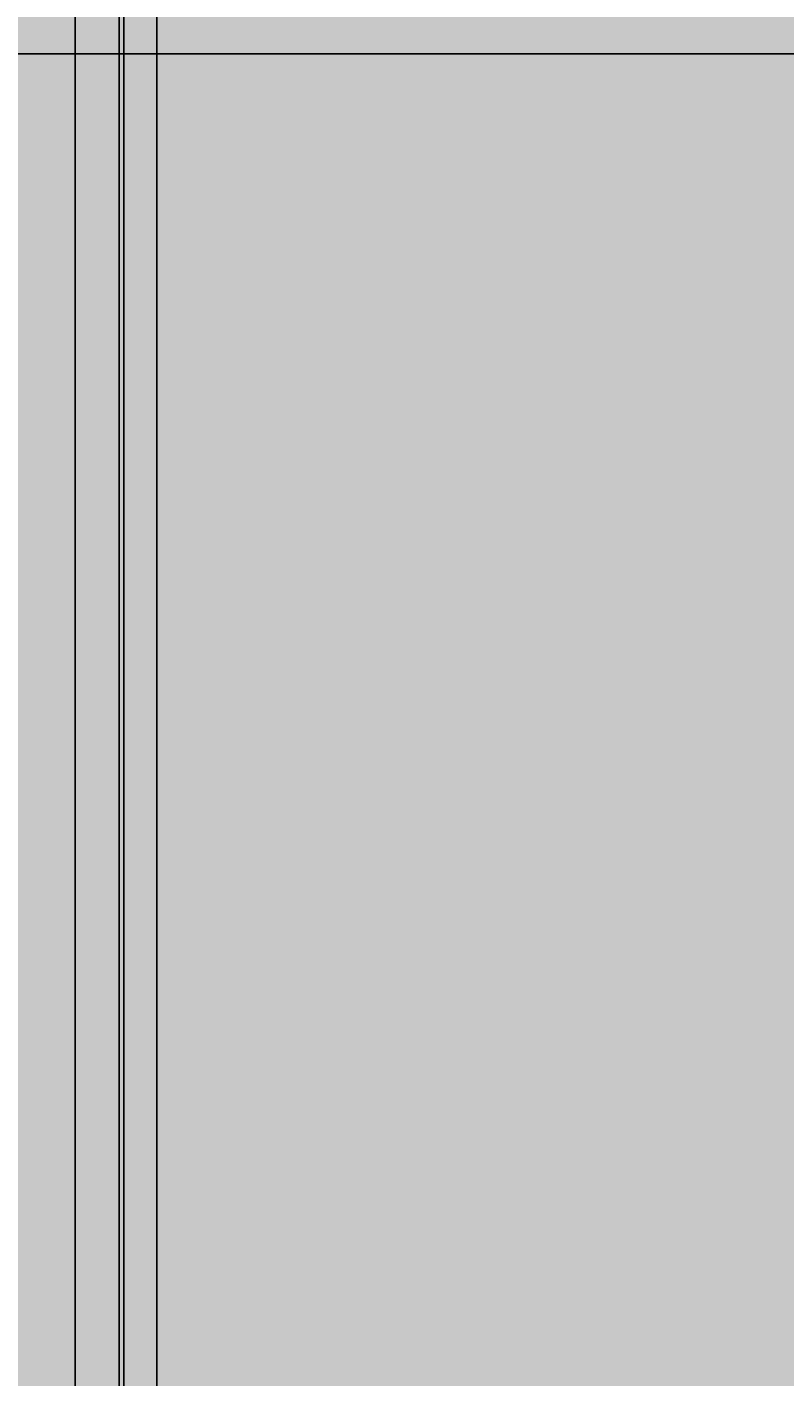
# Model space of a CAD drawing. Units: feet. Extents: x 2695 to 2912, y 795 to 1139.
# Tile 24 of 83: x 2808 to 2825, y 845 to 875. Entities that reach past the tile are written whole.
import ezdxf

# ---------------------------------------------------------------- set-up
doc = ezdxf.new("R2010")
doc.units = ezdxf.units.FT
for name, color, linetype, lineweight in [('A-ANNO-DIMS', 2, 'Continuous', 18), ('A-DOOR', 3, 'Continuous', 25), ('A-DOOR-PATT', 33, 'Continuous', 13)]:
    doc.layers.add(name, color=color, linetype=linetype, lineweight=lineweight)
doc.styles.get("Standard").update_dxf_attribs({"font": 'arial.ttf'})
doc.dimstyles.get("Standard").update_dxf_attribs({"dimtxt": 0.18, "dimasz": 0.18, "dimexe": 0.18, "dimexo": 0.0625, "dimgap": 0.09, "dimtad": 0, "dimtih": 1, "dimtoh": 1, "dimdec": 1, "dimzin": 0, "dimdsep": 46, "dimlunit": 3, "dimtxsty": 'Standard', "dimcen": 0.09, "dimadec": 0, "dimazin": 0, "dimtfac": 1, "dimtdec": 1, "dimtofl": 0, "dimtmove": 0, "dimatfit": 3, "dimfxl": 1, "dimtolj": 1, "dimtzin": 0, "dimarcsym": 0})

# ---------------------------------------------------------------- blocks, each defined once
blk = doc.blocks.new('*D13')
at = {"layer": 'A-ANNO-DIMS', "color": 0, "lineweight": -2, "transparency": 16777216}
for p, q in [((2758.214, 874.857), (2911.424, 874.857)), ((2911.244, 874.677), (2911.244, 843.076)), ((2911.244, 811.111), (2911.244, 842.712)), ((2890.699, 810.931), (2911.424, 810.931))]:
    blk.add_line(p, q, dxfattribs=at)
at = {"layer": 'A-ANNO-DIMS', "color": 0, "transparency": 16777216}
for points in [[(2911.214, 874.677), (2911.274, 874.677), (2911.244, 874.857)], [(2911.214, 811.111), (2911.274, 811.111), (2911.244, 810.931)]]:
    blk.add_solid(points, dxfattribs=at)
at = {"layer": 'Defpoints', "color": 0, "transparency": 16777216}
for p in [(2758.151, 874.857), (2911.244, 874.857), (2890.636, 810.931)]:
    blk.add_point(p, dxfattribs=at)
at = {"layer": 'A-ANNO-DIMS', "color": 0, "transparency": 16777216, "insert": (2911.244, 842.894), "char_height": 0.18, "attachment_point": 5}
blk.add_mtext('\\A1;63.93', dxfattribs=at)
blk = doc.blocks.new('*D14')
at = {"layer": 'A-ANNO-DIMS', "color": 0, "lineweight": -2, "transparency": 16777216}
for p, q in [((2838.439, 905.514), (2911.424, 905.514)), ((2911.244, 905.334), (2911.244, 890.368)), ((2911.244, 875.037), (2911.244, 890.004)), ((2758.214, 874.857), (2911.424, 874.857))]:
    blk.add_line(p, q, dxfattribs=at)
at = {"layer": 'A-ANNO-DIMS', "color": 0, "transparency": 16777216}
for points in [[(2911.214, 905.334), (2911.274, 905.334), (2911.244, 905.514)], [(2911.214, 875.037), (2911.274, 875.037), (2911.244, 874.857)]]:
    blk.add_solid(points, dxfattribs=at)
at = {"layer": 'Defpoints', "color": 0, "transparency": 16777216}
for p in [(2838.377, 905.514), (2911.244, 905.514), (2758.151, 874.857)]:
    blk.add_point(p, dxfattribs=at)
at = {"layer": 'A-ANNO-DIMS', "color": 0, "transparency": 16777216, "insert": (2911.244, 890.186), "char_height": 0.18, "attachment_point": 5}
blk.add_mtext('\\A1;30.66', dxfattribs=at)
blk = doc.blocks.new('*D52')
at = {"layer": 'A-ANNO-DIMS', "color": 0, "lineweight": -2, "transparency": 16777216}
for p, q in [((2810.041, 936.868), (2810.041, 794.976)), ((2810.789, 936.868), (2810.789, 794.976)), ((2809.861, 795.156), (2809.681, 795.156)), ((2810.969, 795.156), (2811.149, 795.156))]:
    blk.add_line(p, q, dxfattribs=at)
at = {"layer": 'A-ANNO-DIMS', "color": 0, "transparency": 16777216}
for points in [[(2809.861, 795.186), (2809.861, 795.126), (2810.041, 795.156)], [(2810.969, 795.186), (2810.969, 795.126), (2810.789, 795.156)]]:
    blk.add_solid(points, dxfattribs=at)
at = {"layer": 'Defpoints', "color": 0, "transparency": 16777216}
for p in [(2810.041, 936.931), (2810.789, 936.931), (2810.789, 795.156)]:
    blk.add_point(p, dxfattribs=at)
at = {"layer": 'A-ANNO-DIMS', "color": 0, "transparency": 16777216, "insert": (2810.415, 795.156), "char_height": 0.18, "attachment_point": 5}
blk.add_mtext('\\A1;0.75', dxfattribs=at)

msp = doc.modelspace()

# ---------------------------------------------------------------- hatches: boundary and pattern name
at = {"layer": 'A-DOOR-PATT'}
h = msp.add_hatch(color=256, dxfattribs=at)
h.set_gradient(color1=(211, 185, 150), color2=(211, 185, 150))
h.paths.add_polyline_path([(2805.9398, 905.5143), (2773.5029, 905.5143), (2773.5029, 810.9306), (2776.4999, 810.9306), (2776.4999, 902.5174), (2802.9429, 902.5174), (2802.9429, 810.9306), (2805.9398, 810.9306)])
h.paths.add_polyline_path([(2803.9681, 874.1057), (2805.0538, 874.1057), (2805.0538, 846.2857), (2803.9681, 846.2857)], flags=16)
h.paths.add_polyline_path([(2838.3767, 905.5143), (2805.9398, 905.5143), (2805.9398, 810.9306), (2808.9368, 810.9306), (2808.9368, 902.5174), (2835.3798, 902.5174), (2835.3798, 810.9306), (2838.3767, 810.9306)])
h = msp.add_hatch(color=256, dxfattribs=at)
h.set_gradient(color1=(211, 185, 150), color2=(211, 185, 150))
h.paths.add_polyline_path([(2777.5029, 901.5143), (2801.9398, 901.5143), (2801.9398, 810.9306), (2802.9429, 810.9306), (2802.9429, 902.5174), (2776.4999, 902.5174), (2776.4999, 810.9306), (2777.5029, 810.9306)])
h.paths.add_polyline_path([(2809.9398, 901.5143), (2834.3767, 901.5143), (2834.3767, 810.9306), (2835.3798, 810.9306), (2835.3798, 902.5174), (2808.9368, 902.5174), (2808.9368, 810.9306), (2809.9398, 810.9306)])
h = msp.add_hatch(color=256, dxfattribs=at)
h.set_gradient(color1=(173, 221, 247), color2=(173, 221, 247))
h.paths.add_polyline_path([(2801.9398, 901.5143), (2777.5029, 901.5143), (2777.5029, 810.9306), (2801.9398, 810.9306)])
h.paths.add_polyline_path([(2834.3767, 901.5143), (2809.9398, 901.5143), (2809.9398, 810.9306), (2834.3767, 810.9306)])

# ---------------------------------------------------------------- linework, layer by layer
at = {"layer": 'A-DOOR'}
for points in [[(2835.3798, 810.9306), (2835.3798, 902.5174), (2808.9368, 902.5174), (2808.9368, 810.9306)], [(2834.3767, 810.9306), (2834.3767, 901.5143), (2809.9398, 901.5143), (2809.9398, 810.9306)]]:
    msp.add_lwpolyline(points, dxfattribs=at)
for points in [[(2808.9368, 902.5174), (2835.3798, 902.5174), (2835.3798, 810.9306), (2808.9368, 810.9306)], [(2809.9398, 901.5143), (2834.3767, 901.5143), (2834.3767, 810.9306), (2809.9398, 810.9306)]]:
    msp.add_lwpolyline(points, close=True, dxfattribs=at)

# ---------------------------------------------------------------- dimensions: what is measured, and where the dimension line sits
at = {"layer": 'A-ANNO-DIMS'}
dim = msp.add_linear_dim(base=(2810.7893, 795.1556), p1=(2810.0407, 936.9306), p2=(2810.7893, 936.9306), dimstyle='Standard', override={"dimdec": 2, "dimlfac": 1, "dimrnd": 0, "dimzin": 0, "dimdsep": 46, "dimlunit": 2}, dxfattribs=at)
dim.commit()
dim.dimension.update_dxf_attribs({"geometry": '*D52', "text_midpoint": (2810.415, 795.1556)})
for base, p1, p2, picture, middle in [((2911.2444, 905.5143), (2758.1515, 874.8571), (2838.3767, 905.5143), '*D14', (2911.2444, 890.1857)), ((2911.2444, 874.8571), (2890.6361, 810.9306), (2758.1515, 874.8571), '*D13', (2911.2444, 842.8938))]:
    dim = msp.add_linear_dim(base=base, p1=p1, p2=p2, angle=90, dimstyle='Standard', override={"dimdec": 2, "dimlfac": 1, "dimrnd": 0, "dimzin": 0, "dimdsep": 46, "dimlunit": 2}, dxfattribs=at)
    dim.commit()
    dim.dimension.update_dxf_attribs({"geometry": picture, "text_midpoint": middle})

doc.saveas('drawing.dxf')
